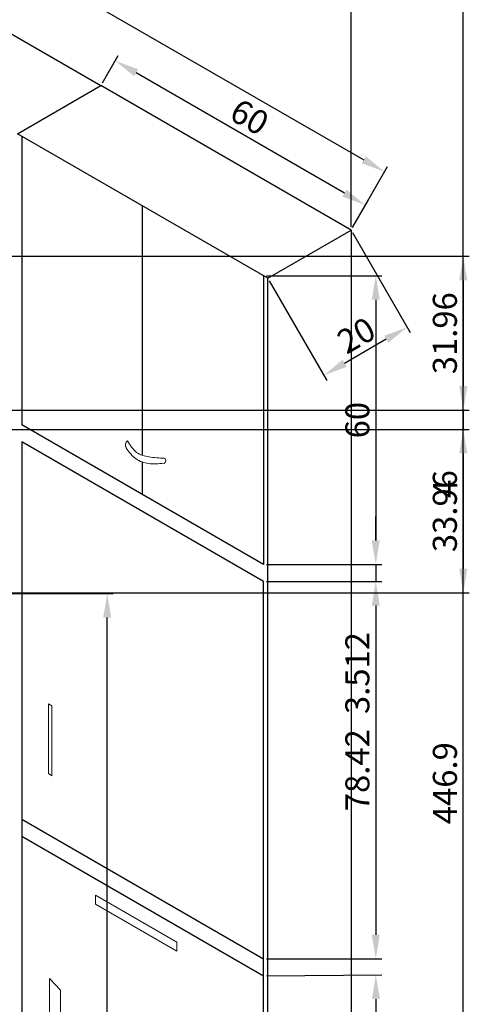
# Model space of a CAD drawing. Units: centimetres. Extents: x 2148 to 2649, y 4226 to 4785.
# Tile 5 of 6: x 2555 to 2649, y 4445 to 4649. Entities that reach past the tile are written whole.
import ezdxf

# ---------------------------------------------------------------- set-up
doc = ezdxf.new("R2010")
doc.units = ezdxf.units.CM
for name, color, linetype, lineweight in [('A-ANNO-DIMS', 63, 'Continuous', 18), ('A-FLOR-CASE', 21, 'Continuous', 25), ('A-FLOR-CASE-HDW', 21, 'Continuous', 18), ('A-FLOR-CASE-TALL', 30, 'Continuous', 30)]:
    doc.layers.add(name, color=color, linetype=linetype, lineweight=lineweight)
doc.styles.get("Standard").update_dxf_attribs({"font": 'arial.ttf'})
doc.dimstyles.new('ISO-25', dxfattribs={"dimtxt": 5, "dimasz": 5, "dimexe": 1.25, "dimexo": 0.625, "dimtad": 1, "dimdec": 1, "dimtxsty": 'Standard', "dimcen": 2.5, "dimadec": 0, "dimazin": 0, "dimtfac": 1, "dimtdec": 1, "dimtmove": 0, "dimatfit": 3, "dimfxl": 1, "dimarcsym": 0})

# ---------------------------------------------------------------- blocks, each defined once
blk = doc.blocks.new('*D6')
at = {"layer": 'A-ANNO-DIMS', "color": 0, "lineweight": -2, "transparency": 16777216}
for p, q in [((2436.59, 4714.79), (2443.88, 4727.41)), ((2447.59, 4723.83), (2626.86, 4620.33)), ((2624.52, 4606.29), (2631.81, 4618.91))]:
    blk.add_line(p, q, dxfattribs=at)
at = {"layer": 'A-ANNO-DIMS', "color": 0, "transparency": 16777216}
for points in [[(2448.01, 4724.55), (2447.17, 4723.11), (2443.26, 4726.33)], [(2627.27, 4621.05), (2626.44, 4619.61), (2631.19, 4617.83)]]:
    blk.add_solid(points, dxfattribs=at)
at = {"layer": 'Defpoints', "color": 0, "transparency": 16777216}
for p in [(2436.28, 4714.24), (2631.19, 4617.83), (2624.21, 4605.74)]:
    blk.add_point(p, dxfattribs=at)
at = {"layer": 'A-ANNO-DIMS', "color": 0, "transparency": 16777216, "insert": (2538.79, 4674.79), "char_height": 5, "attachment_point": 5, "rotation": 330}
blk.add_mtext('217', dxfattribs=at)
blk = doc.blocks.new('*D7')
at = {"layer": 'A-ANNO-DIMS', "color": 0, "lineweight": -2, "transparency": 16777216}
for p, q in [((2572.56, 4636.29), (2575.85, 4641.99)), ((2622.86, 4613.4), (2579.56, 4638.4)), ((2624.52, 4606.29), (2627.81, 4611.99))]:
    blk.add_line(p, q, dxfattribs=at)
at = {"layer": 'A-ANNO-DIMS', "color": 0, "transparency": 16777216}
for points in [[(2579.97, 4639.13), (2579.14, 4637.68), (2575.23, 4640.9)], [(2623.27, 4614.13), (2622.44, 4612.68), (2627.19, 4610.9)]]:
    blk.add_solid(points, dxfattribs=at)
at = {"layer": 'Defpoints', "color": 0, "transparency": 16777216}
for p in [(2575.23, 4640.9), (2572.25, 4635.74), (2624.21, 4605.74)]:
    blk.add_point(p, dxfattribs=at)
at = {"layer": 'A-ANNO-DIMS', "color": 0, "transparency": 16777216, "insert": (2602.8, 4628.66), "char_height": 5, "attachment_point": 5, "rotation": 330}
blk.add_mtext('60', dxfattribs=at)
blk = doc.blocks.new('*D30')
at = {"layer": 'A-ANNO-DIMS', "color": 0, "lineweight": -2, "transparency": 16777216}
for p, q in [((2534.71, 4530.22), (2574.8, 4530.22)), ((2573.55, 4272.15), (2573.55, 4525.22)), ((2534.71, 4267.15), (2574.8, 4267.15))]:
    blk.add_line(p, q, dxfattribs=at)
at = {"layer": 'A-ANNO-DIMS', "color": 0, "transparency": 16777216}
for points in [[(2572.71, 4525.22), (2574.38, 4525.22), (2573.55, 4530.22)], [(2572.71, 4272.15), (2574.38, 4272.15), (2573.55, 4267.15)]]:
    blk.add_solid(points, dxfattribs=at)
at = {"layer": 'Defpoints', "color": 0, "transparency": 16777216}
for p in [(2534.09, 4530.22), (2573.55, 4530.22), (2534.09, 4267.15)]:
    blk.add_point(p, dxfattribs=at)
at = {"layer": 'A-ANNO-DIMS', "color": 0, "transparency": 16777216, "insert": (2569.64, 4398.69), "char_height": 5, "attachment_point": 5, "rotation": 90}
blk.add_mtext('ISLAND (PROJ.) 263', dxfattribs=at)
blk = doc.blocks.new('*D42')
at = {"layer": 'A-ANNO-DIMS', "color": 0, "lineweight": -2, "transparency": 16777216}
for p, q in [((2305.27, 4600.28), (2648.78, 4600.28)), ((2647.53, 4595.28), (2647.53, 4573.32)), ((2305.27, 4568.32), (2648.78, 4568.32))]:
    blk.add_line(p, q, dxfattribs=at)
at = {"layer": 'A-ANNO-DIMS', "color": 0, "transparency": 16777216}
for points in [[(2646.7, 4595.28), (2648.37, 4595.28), (2647.53, 4600.28)], [(2646.7, 4573.32), (2648.37, 4573.32), (2647.53, 4568.32)]]:
    blk.add_solid(points, dxfattribs=at)
at = {"layer": 'Defpoints', "color": 0, "transparency": 16777216}
for p in [(2304.65, 4600.28), (2304.65, 4568.32), (2647.53, 4568.32)]:
    blk.add_point(p, dxfattribs=at)
at = {"layer": 'A-ANNO-DIMS', "color": 0, "transparency": 16777216, "insert": (2644.35, 4584.3), "char_height": 5, "attachment_point": 5, "rotation": 90}
blk.add_mtext('31.96', dxfattribs=at)
blk = doc.blocks.new('*D43')
at = {"layer": 'A-ANNO-DIMS', "color": 0, "lineweight": -2, "transparency": 16777216}
for p, q in [((2647.53, 4573.32), (2647.53, 4578.32)), ((2305.27, 4568.32), (2648.78, 4568.32)), ((2647.53, 4568.32), (2647.53, 4564.32)), ((2305.27, 4564.32), (2648.78, 4564.32)), ((2647.53, 4559.32), (2647.53, 4549.61))]:
    blk.add_line(p, q, dxfattribs=at)
at = {"layer": 'A-ANNO-DIMS', "color": 0, "transparency": 16777216}
for points in [[(2646.7, 4573.32), (2648.37, 4573.32), (2647.53, 4568.32)], [(2646.7, 4559.32), (2648.37, 4559.32), (2647.53, 4564.32)]]:
    blk.add_solid(points, dxfattribs=at)
at = {"layer": 'Defpoints', "color": 0, "transparency": 16777216}
for p in [(2304.65, 4568.32), (2304.65, 4564.32), (2647.53, 4564.32)]:
    blk.add_point(p, dxfattribs=at)
at = {"layer": 'A-ANNO-DIMS', "color": 0, "transparency": 16777216, "insert": (2644.41, 4551.97), "char_height": 5, "attachment_point": 5, "rotation": 90}
blk.add_mtext('4', dxfattribs=at)
blk = doc.blocks.new('*D44')
at = {"layer": 'A-ANNO-DIMS', "color": 0, "lineweight": -2, "transparency": 16777216}
for p, q in [((2305.27, 4564.32), (2648.78, 4564.32)), ((2647.53, 4559.32), (2647.53, 4535.36)), ((2305.27, 4530.36), (2648.78, 4530.36))]:
    blk.add_line(p, q, dxfattribs=at)
at = {"layer": 'A-ANNO-DIMS', "color": 0, "transparency": 16777216}
for points in [[(2646.7, 4559.32), (2648.37, 4559.32), (2647.53, 4564.32)], [(2646.7, 4535.36), (2648.37, 4535.36), (2647.53, 4530.36)]]:
    blk.add_solid(points, dxfattribs=at)
at = {"layer": 'Defpoints', "color": 0, "transparency": 16777216}
for p in [(2304.65, 4564.32), (2304.65, 4530.36), (2647.53, 4530.36)]:
    blk.add_point(p, dxfattribs=at)
at = {"layer": 'A-ANNO-DIMS', "color": 0, "transparency": 16777216, "insert": (2644.35, 4547.34), "char_height": 5, "attachment_point": 5, "rotation": 90}
blk.add_mtext('33.96', dxfattribs=at)
blk = doc.blocks.new('*D50')
at = {"layer": 'A-ANNO-DIMS', "color": 0, "lineweight": -2, "transparency": 16777216}
for p, q in [((2178.26, 4588.31), (2178.26, 4738.82)), ((2624.21, 4606.37), (2624.21, 4738.82)), ((2183.26, 4737.57), (2619.21, 4737.57))]:
    blk.add_line(p, q, dxfattribs=at)
at = {"layer": 'A-ANNO-DIMS', "color": 0, "transparency": 16777216}
for points in [[(2183.26, 4738.4), (2183.26, 4736.74), (2178.26, 4737.57)], [(2619.21, 4738.4), (2619.21, 4736.74), (2624.21, 4737.57)]]:
    blk.add_solid(points, dxfattribs=at)
at = {"layer": 'Defpoints', "color": 0, "transparency": 16777216}
for p in [(2624.21, 4737.57), (2624.21, 4605.74), (2178.26, 4587.69)]:
    blk.add_point(p, dxfattribs=at)
at = {"layer": 'A-ANNO-DIMS', "color": 0, "transparency": 16777216, "insert": (2401.23, 4740.75), "char_height": 5, "attachment_point": 5}
blk.add_mtext('445.95', dxfattribs=at)
blk = doc.blocks.new('*D51')
at = {"layer": 'A-ANNO-DIMS', "color": 0, "lineweight": -2, "transparency": 16777216}
for p, q in [((2436.91, 4714.24), (2648.78, 4714.24)), ((2647.53, 4272.37), (2647.53, 4709.24)), ((2409.81, 4267.37), (2648.78, 4267.37))]:
    blk.add_line(p, q, dxfattribs=at)
at = {"layer": 'A-ANNO-DIMS', "color": 0, "transparency": 16777216}
for points in [[(2646.7, 4709.24), (2648.37, 4709.24), (2647.53, 4714.24)], [(2646.7, 4272.37), (2648.37, 4272.37), (2647.53, 4267.37)]]:
    blk.add_solid(points, dxfattribs=at)
at = {"layer": 'Defpoints', "color": 0, "transparency": 16777216}
for p in [(2436.28, 4714.24), (2647.53, 4714.24), (2409.18, 4267.37)]:
    blk.add_point(p, dxfattribs=at)
at = {"layer": 'A-ANNO-DIMS', "color": 0, "transparency": 16777216, "insert": (2644.36, 4490.81), "char_height": 5, "attachment_point": 5, "rotation": 90}
blk.add_mtext('446.9', dxfattribs=at)
blk = doc.blocks.new('*D60')
at = {"layer": 'A-ANNO-DIMS', "color": 0, "lineweight": -2, "transparency": 16777216}
for p, q in [((2624.52, 4605.2), (2636.5, 4584.46)), ((2607.2, 4595.2), (2619.18, 4574.46)), ((2631.54, 4583.04), (2622.88, 4578.04))]:
    blk.add_line(p, q, dxfattribs=at)
at = {"layer": 'A-ANNO-DIMS', "color": 0, "transparency": 16777216}
for points in [[(2631.12, 4583.77), (2631.96, 4582.32), (2635.87, 4585.54)], [(2622.46, 4578.77), (2623.3, 4577.32), (2618.55, 4575.54)]]:
    blk.add_solid(points, dxfattribs=at)
at = {"layer": 'Defpoints', "color": 0, "transparency": 16777216}
for p in [(2624.21, 4605.74), (2606.89, 4595.74), (2618.55, 4575.54)]:
    blk.add_point(p, dxfattribs=at)
at = {"layer": 'A-ANNO-DIMS', "color": 0, "transparency": 16777216, "insert": (2625.62, 4583.3), "char_height": 5, "attachment_point": 5, "rotation": 30}
blk.add_mtext('20', dxfattribs=at)
blk = doc.blocks.new('*D62')
at = {"layer": 'A-ANNO-DIMS', "color": 0, "lineweight": -2, "transparency": 16777216}
for p, q in [((2606.65, 4596.24), (2630.6, 4596.24)), ((2629.35, 4591.24), (2629.35, 4541.24)), ((2606.65, 4536.24), (2630.6, 4536.24))]:
    blk.add_line(p, q, dxfattribs=at)
at = {"layer": 'A-ANNO-DIMS', "color": 0, "transparency": 16777216}
for points in [[(2628.51, 4591.24), (2630.18, 4591.24), (2629.35, 4596.24)], [(2628.51, 4541.24), (2630.18, 4541.24), (2629.35, 4536.24)]]:
    blk.add_solid(points, dxfattribs=at)
at = {"layer": 'Defpoints', "color": 0, "transparency": 16777216}
for p in [(2606.02, 4596.24), (2606.02, 4536.24), (2629.35, 4536.24)]:
    blk.add_point(p, dxfattribs=at)
at = {"layer": 'A-ANNO-DIMS', "color": 0, "transparency": 16777216, "insert": (2626.17, 4566.24), "char_height": 5, "attachment_point": 5, "rotation": 90}
blk.add_mtext('60', dxfattribs=at)
blk = doc.blocks.new('*D63')
at = {"layer": 'A-ANNO-DIMS', "color": 0, "lineweight": -2, "transparency": 16777216}
for p, q in [((2629.35, 4541.24), (2629.35, 4546.24)), ((2606.65, 4536.24), (2630.6, 4536.24)), ((2629.35, 4536.24), (2629.35, 4532.73)), ((2606.65, 4532.73), (2630.6, 4532.73)), ((2629.35, 4527.73), (2629.35, 4504.66))]:
    blk.add_line(p, q, dxfattribs=at)
at = {"layer": 'A-ANNO-DIMS', "color": 0, "transparency": 16777216}
for points in [[(2628.51, 4541.24), (2630.18, 4541.24), (2629.35, 4536.24)], [(2628.51, 4527.73), (2630.18, 4527.73), (2629.35, 4532.73)]]:
    blk.add_solid(points, dxfattribs=at)
at = {"layer": 'Defpoints', "color": 0, "transparency": 16777216}
for p in [(2606.02, 4536.24), (2606.02, 4532.73), (2629.35, 4532.73)]:
    blk.add_point(p, dxfattribs=at)
at = {"layer": 'A-ANNO-DIMS', "color": 0, "transparency": 16777216, "insert": (2626.17, 4513.7), "char_height": 5, "attachment_point": 5, "rotation": 90}
blk.add_mtext('3.512', dxfattribs=at)
blk = doc.blocks.new('*D64')
at = {"layer": 'A-ANNO-DIMS', "color": 0, "lineweight": -2, "transparency": 16777216}
for p, q in [((2606.65, 4532.73), (2630.6, 4532.73)), ((2629.35, 4527.73), (2629.35, 4459.31)), ((2606.65, 4454.31), (2630.6, 4454.31))]:
    blk.add_line(p, q, dxfattribs=at)
at = {"layer": 'A-ANNO-DIMS', "color": 0, "transparency": 16777216}
for points in [[(2628.51, 4527.73), (2630.18, 4527.73), (2629.35, 4532.73)], [(2628.51, 4459.31), (2630.18, 4459.31), (2629.35, 4454.31)]]:
    blk.add_solid(points, dxfattribs=at)
at = {"layer": 'Defpoints', "color": 0, "transparency": 16777216}
for p in [(2606.02, 4532.73), (2606.02, 4454.31), (2629.35, 4454.31)]:
    blk.add_point(p, dxfattribs=at)
at = {"layer": 'A-ANNO-DIMS', "color": 0, "transparency": 16777216, "insert": (2626.17, 4493.52), "char_height": 5, "attachment_point": 5, "rotation": 90}
blk.add_mtext('78.42', dxfattribs=at)
blk = doc.blocks.new('*D65')
at = {"layer": 'A-ANNO-DIMS', "color": 0, "lineweight": -2, "transparency": 16777216}
for p, q in [((2606.65, 4450.81), (2630.6, 4450.98)), ((2629.38, 4445.97), (2630.18, 4335.42)), ((2607.51, 4330.26), (2631.46, 4330.43))]:
    blk.add_line(p, q, dxfattribs=at)
at = {"layer": 'A-ANNO-DIMS', "color": 0, "transparency": 16777216}
for points in [[(2630.22, 4445.98), (2628.55, 4445.97), (2629.35, 4450.97)], [(2631.01, 4335.43), (2629.34, 4335.42), (2630.21, 4330.42)]]:
    blk.add_solid(points, dxfattribs=at)
at = {"layer": 'Defpoints', "color": 0, "transparency": 16777216}
for p in [(2606.02, 4450.81), (2606.89, 4330.26), (2630.21, 4330.42)]:
    blk.add_point(p, dxfattribs=at)
at = {"layer": 'A-ANNO-DIMS', "color": 0, "transparency": 16777216, "insert": (2632.96, 4390.72), "char_height": 5, "attachment_point": 5, "rotation": 270.4116}
blk.add_mtext('120.55', dxfattribs=at)

msp = doc.modelspace()

# ---------------------------------------------------------------- linework, layer by layer
at = {"layer": 'A-FLOR-CASE'}
msp.add_line((2513.8379, 4669.4674), (2572.2471, 4635.7447), dxfattribs=at)
at = {"layer": 'A-FLOR-CASE-HDW'}
for p, q in [((2561.3409, 4492.8465), (2561.3409, 4507.2812)), ((2561.3409, 4507.2812), (2562.0627, 4506.8645)), ((2562.0627, 4506.8645), (2562.0627, 4492.3515)), ((2562.0627, 4492.3515), (2561.3409, 4492.8465)), ((2571.0854, 4467.5355), (2588.0196, 4457.7585)), ((2571.0854, 4467.5355), (2571.0854, 4465.6819)), ((2588.0196, 4455.9049), (2571.0854, 4465.6819)), ((2588.0196, 4457.7585), (2588.0196, 4455.9049)), ((2561.585, 4450.2388), (2561.585, 4382.7199)), ((2563.8432, 4447.8355), (2561.585, 4450.2388)), ((2563.8432, 4381.4161), (2563.8432, 4447.8355))]:
    msp.add_line(p, q, dxfattribs=at)
for centre, radius, start, end in [((2578.5902, 4561.0066), 1.2562, 131.346915, 205.051704), ((2585.1709, 4557.8346), 0.5756, 282.11805, 62.307207)]:
    msp.add_arc(centre, radius, start, end, dxfattribs=at)
for points, knots in [([(2577.7603, 4561.9496), (2578.3061, 4561.0398), (2579.3398, 4559.3169), (2582.4063, 4558.4562), (2584.3747, 4558.3835), (2585.4384, 4558.3443)], [0, 0, 0, 0, 3.06315218, 5.80087049, 9.01902056, 9.01902056, 9.01902056, 9.01902056]), ([(2577.4522, 4560.4747), (2578.0789, 4559.6141), (2579.2555, 4557.9985), (2582.2693, 4557.0042), (2584.2366, 4557.1785), (2585.2917, 4557.2719)], [0, 0, 0, 0, 3.12002973, 5.85774805, 9.02488051, 9.02488051, 9.02488051, 9.02488051])]:
    msp.add_open_spline(points, degree=3, knots=knots, dxfattribs=at)
at = {"layer": 'A-FLOR-CASE-TALL'}
for p, q in [((2554.9266, 4625.7447), (2572.2471, 4635.7447)), ((2624.2087, 4605.7447), (2572.2471, 4635.7447)), ((2606.8882, 4595.7447), (2554.9266, 4625.7447)), ((2555.7927, 4625.2447), (2555.7927, 4565.2447)), ((2580.9074, 4558.9281), (2580.9074, 4610.7447)), ((2606.8882, 4595.7447), (2624.2087, 4605.7447)), ((2624.2087, 4605.7447), (2624.2087, 4330.7447)), ((2606.0221, 4596.2447), (2606.0221, 4536.2447)), ((2606.8882, 4320.7447), (2606.8882, 4595.7447)), ((2606.0221, 4536.2447), (2555.7927, 4565.2447)), ((2606.0221, 4532.7324), (2555.7927, 4561.7324)), ((2555.7927, 4561.7324), (2555.7927, 4350.2447)), ((2580.9074, 4550.7447), (2580.9074, 4557.5154)), ((2606.0221, 4321.2447), (2606.0221, 4532.7324)), ((2555.7927, 4483.3081), (2606.0221, 4454.3081)), ((2555.7927, 4479.8052), (2606.0221, 4450.8052))]:
    msp.add_line(p, q, dxfattribs=at)

# ---------------------------------------------------------------- dimensions: what is measured, and where the dimension line sits
at = {"layer": 'A-ANNO-DIMS'}
dim = msp.add_linear_dim(base=(2624.2087, 4737.5697), p1=(2178.2568, 4587.6856), p2=(2624.2087, 4605.7447), dimstyle='ISO-25', override={"dimdec": 2, "dimlfac": 1, "dimrnd": 0, "dimzin": 0, "dimdsep": 46, "dimlunit": 2}, dxfattribs=at)
dim.commit()
dim.dimension.update_dxf_attribs({"geometry": '*D50', "text_midpoint": (2401.2328, 4740.7476)})
for p1, p2, distance, picture, middle in [((2436.2812, 4714.2447), (2624.2087, 4605.7447), 13.9546, '*D6', (2538.7898, 4674.795)), ((2624.2087, 4605.7447), (2572.2471, 4635.7447), -5.9576, '*D7', (2602.7957, 4628.6563))]:
    dim = msp.add_aligned_dim(p1=p1, p2=p2, distance=distance, dimstyle='ISO-25', override={"dimclrd": 0, "dimclre": 0, "dimclrt": 0}, dxfattribs=at)
    dim.commit()
    dim.dimension.update_dxf_attribs({"geometry": picture, "text_midpoint": middle})
for base, p1, p2, angle, override, picture, middle in [((2647.5337, 4714.2447), (2409.1829, 4267.3731), (2436.2812, 4714.2447), 90, {"dimdec": 1, "dimlfac": 1, "dimrnd": 0, "dimzin": 0, "dimdsep": 46, "dimlunit": 2}, '*D51', (2644.3558, 4490.8089)), ((2618.5507, 4575.5447), (2624.2087, 4605.7447), (2606.8882, 4595.7447), 210, {"dimdec": 0, "dimlfac": 1, "dimrnd": 0, "dimzin": 0, "dimdsep": 46, "dimlunit": 2}, '*D60', (2625.622, 4583.2968)), ((2647.5337, 4568.3196), (2304.6453, 4600.2822), (2304.6453, 4568.3196), 90, {"dimdec": 2, "dimlfac": 1, "dimrnd": 0, "dimzin": 0, "dimdsep": 46, "dimlunit": 2}, '*D42', (2644.3541, 4584.3009)), ((2629.3471, 4536.2447), (2606.0221, 4596.2447), (2606.0221, 4536.2447), 270, {"dimdec": 0, "dimlfac": 1, "dimrnd": 0, "dimzin": 0, "dimdsep": 46, "dimlunit": 2}, '*D62', (2626.1693, 4566.2447)), ((2647.5337, 4564.3196), (2304.6453, 4568.3196), (2304.6453, 4564.3196), 90, {"dimdec": 0, "dimlfac": 1, "dimrnd": 0, "dimzin": 0, "dimdsep": 46, "dimlunit": 2}, '*D43', (2644.4087, 4551.9654)), ((2647.5337, 4530.357), (2304.6453, 4564.3196), (2304.6453, 4530.357), 90, {"dimdec": 2, "dimlfac": 1, "dimrnd": 0, "dimzin": 0, "dimdsep": 46, "dimlunit": 2}, '*D44', (2644.3541, 4547.3383)), ((2629.3471, 4532.7324), (2606.0221, 4536.2447), (2606.0221, 4532.7324), 270, {"dimdec": 3, "dimlfac": 1, "dimrnd": 0, "dimzin": 0, "dimdsep": 46, "dimlunit": 2}, '*D63', (2626.1676, 4513.6985)), ((2629.3471, 4454.3081), (2606.0221, 4532.7324), (2606.0221, 4454.3081), 270, {"dimdec": 2, "dimlfac": 1, "dimrnd": 0, "dimzin": 0, "dimdsep": 46, "dimlunit": 2}, '*D64', (2626.1693, 4493.5203)), ((2630.2126, 4330.4235), (2606.0221, 4450.8052), (2606.8882, 4330.2559), 270.411605, {"dimdec": 2, "dimlfac": 1, "dimrnd": 0, "dimzin": 0, "dimdsep": 46, "dimlunit": 2}, '*D65', (2632.9573, 4390.721))]:
    dim = msp.add_linear_dim(base=base, p1=p1, p2=p2, angle=angle, dimstyle='ISO-25', override=override, dxfattribs=at)
    dim.commit()
    dim.dimension.update_dxf_attribs({"geometry": picture, "text_midpoint": middle})
dim = msp.add_linear_dim(base=(2573.5478, 4530.2236), p1=(2534.0868, 4267.1498), p2=(2534.0868, 4530.2236), angle=90, text='ISLAND (PROJ.) <>', dimstyle='ISO-25', override={"dimdec": 0, "dimlfac": 1, "dimrnd": 0, "dimzin": 0, "dimdsep": 46, "dimlunit": 2}, dxfattribs=at)
dim.commit()
dim.dimension.update_dxf_attribs({"geometry": '*D30', "text_midpoint": (2569.6435, 4398.6867)})

doc.saveas('drawing.dxf')
